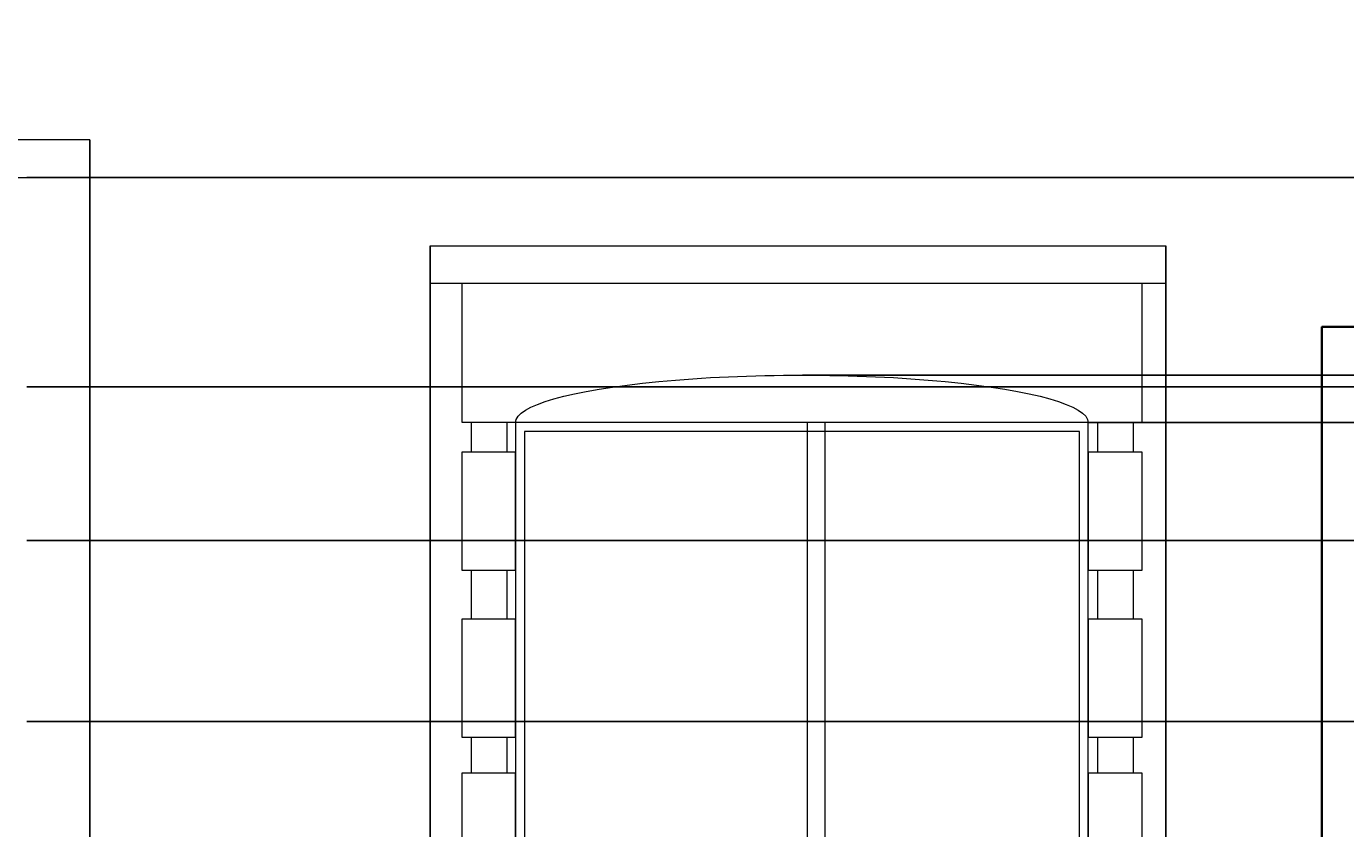
# Model space of a CAD drawing. Units: inches. Extents: x 69 to 650, y -16 to 573.
# Tile 20 of 26: x 383 to 531, y 308 to 398. Entities that reach past the tile are written whole.
import ezdxf

# ---------------------------------------------------------------- set-up
doc = ezdxf.new("R2010")
doc.units = ezdxf.units.IN
doc.header["$MEASUREMENT"] = 0
for name, color, linetype, lineweight in [('A-ANNO-DIMS', 2, 'Continuous', 18), ('A-GLAZ', 4, 'Continuous', 18), ('A-WALL', 7, 'Continuous', 35)]:
    doc.layers.add(name, color=color, linetype=linetype, lineweight=lineweight)
doc.styles.get("Standard").update_dxf_attribs({"font": 'arial.ttf'})
doc.dimstyles.get("Standard").update_dxf_attribs({"dimtxt": 0.8125, "dimasz": 0.18, "dimexe": 0.18, "dimexo": 0.0625, "dimgap": 0.09, "dimtad": 0, "dimtih": 1, "dimtoh": 1, "dimdec": 4, "dimzin": 0, "dimdsep": 46, "dimlunit": 4, "dimtxsty": 'Standard', "dimcen": 0.09, "dimadec": 0, "dimazin": 0, "dimtfac": 1, "dimtdec": 4, "dimtofl": 0, "dimtmove": 0, "dimatfit": 3, "dimfxl": 1, "dimtolj": 1, "dimtzin": 0, "dimarcsym": 0})

# ---------------------------------------------------------------- blocks, each defined once
blk = doc.blocks.new('WIN-ARCH-SURROUND')
for p, q in [((0, 129.06), (0, 124.83)), ((82.63, 129.06), (0, 129.06)), ((82.63, 124.83), (82.63, 129.06)), ((0, 124.83), (82.63, 124.83)), ((2.69, 109.21), (2.69, 124.83)), ((79.05, 109.21), (79.05, 124.83)), ((3.69, 109.21), (2.69, 109.21)), ((3.69, 109.21), (3.69, 105.89)), ((3.69, 109.21), (78.05, 109.21)), ((7.69, 109.21), (7.69, 105.89)), ((8.73, 105.89), (8.73, 109.21)), ((38.31, 109.21), (38.31, 38)), ((40.31, 109.21), (40.31, 38)), ((74.05, 109.21), (74.05, 105.89)), ((78.05, 109.21), (79.05, 109.21)), ((78.05, 109.21), (78.05, 105.89)), ((3.69, 92.64), (3.69, 87.15)), ((7.69, 92.64), (7.69, 87.15)), ((74.05, 92.64), (74.05, 87.15)), ((78.05, 92.64), (78.05, 87.15)), ((3.69, 73.9), (3.69, 69.84)), ((7.69, 73.9), (7.69, 69.84)), ((74.05, 73.9), (74.05, 69.84)), ((78.05, 73.9), (78.05, 69.84)), ((3.69, 56.59), (3.69, 51.51)), ((7.69, 56.59), (7.69, 51.51)), ((74.05, 56.59), (74.05, 51.51)), ((78.05, 56.59), (78.05, 51.51)), ((3.69, 38.26), (3.69, 33.16)), ((7.69, 38.26), (7.69, 33.16)), ((74.05, 38.26), (74.05, 33.16)), ((78.05, 38.26), (78.05, 33.16)), ((3.69, 19.91), (3.69, 0)), ((7.69, 19.91), (7.69, 0)), ((74.05, 19.91), (74.05, 0)), ((78.05, 19.91), (78.05, 0))]:
    blk.add_line(p, q)
for points in [[(8.73, 109.21), (73.05, 109.21), (73.05, 38.26), (8.73, 38.26)], [(9.73, 108.21), (72.05, 108.21), (72.05, 39.26), (9.73, 39.26)], [(2.69, 105.89), (8.73, 105.89), (8.73, 92.64), (2.69, 92.64)], [(73.05, 105.89), (79.1, 105.89), (79.1, 92.64), (73.05, 92.64)], [(2.69, 87.15), (8.73, 87.15), (8.73, 73.9), (2.69, 73.9)], [(73.05, 87.15), (79.1, 87.15), (79.1, 73.9), (73.05, 73.9)], [(2.69, 69.84), (8.73, 69.84), (8.73, 56.59), (2.69, 56.59)], [(73.05, 69.84), (79.1, 69.84), (79.1, 56.59), (73.05, 56.59)], [(2.69, 51.51), (8.73, 51.51), (8.73, 38.26), (2.69, 38.26)], [(73.05, 51.51), (79.1, 51.51), (79.1, 38.26), (73.05, 38.26)], [(2.65, 33.16), (8.69, 33.16), (8.69, 19.91), (2.65, 19.91)], [(73.01, 33.16), (79.06, 33.16), (79.06, 19.91), (73.01, 19.91)]]:
    blk.add_lwpolyline(points, close=True)
blk.add_ellipse((40.89, 109.21), major_axis=(32.16, 0), ratio=0.165597, start_param=6.283185, end_param=9.424778)
blk = doc.blocks.new('*D19')
at = {"layer": 'A-ANNO-DIMS', "color": 0, "lineweight": -2, "transparency": 16777216}
for p, q in [((99.56, 471.72), (99.56, 572.74)), ((99.74, 572.56), (358.57, 572.56)), ((619.38, 572.56), (360.54, 572.56)), ((619.56, 87.99), (619.56, 572.74))]:
    blk.add_line(p, q, dxfattribs=at)
at = {"layer": 'A-ANNO-DIMS', "color": 0, "transparency": 16777216}
for points in [[(99.74, 572.59), (99.74, 572.53), (99.56, 572.56)], [(619.38, 572.59), (619.38, 572.53), (619.56, 572.56)]]:
    blk.add_solid(points, dxfattribs=at)
at = {"layer": 'Defpoints', "color": 0, "transparency": 16777216}
for p in [(619.56, 572.56), (99.56, 471.66), (619.56, 87.93)]:
    blk.add_point(p, dxfattribs=at)
at = {"layer": 'A-ANNO-DIMS', "color": 0, "transparency": 16777216, "insert": (359.56, 572.56), "char_height": 0.812, "attachment_point": 5}
blk.add_mtext('\\A1;520', dxfattribs=at)
blk = doc.blocks.new('*D20')
at = {"layer": 'A-ANNO-DIMS', "color": 0, "lineweight": -2, "transparency": 16777216}
for p, q in [((504.24, 544.16), (648.14, 544.16)), ((647.96, 543.98), (647.96, 304.55)), ((647.96, 64.11), (647.96, 303.54)), ((619.62, 63.93), (648.14, 63.93))]:
    blk.add_line(p, q, dxfattribs=at)
at = {"layer": 'A-ANNO-DIMS', "color": 0, "transparency": 16777216}
for points in [[(647.93, 543.98), (647.99, 543.98), (647.96, 544.16)], [(647.93, 64.11), (647.99, 64.11), (647.96, 63.93)]]:
    blk.add_solid(points, dxfattribs=at)
at = {"layer": 'Defpoints', "color": 0, "transparency": 16777216}
for p in [(504.18, 544.16), (647.96, 544.16), (619.56, 63.93)]:
    blk.add_point(p, dxfattribs=at)
at = {"layer": 'A-ANNO-DIMS', "color": 0, "transparency": 16777216, "insert": (647.96, 304.04), "char_height": 0.812, "attachment_point": 5}
blk.add_mtext('\\A1;480.2', dxfattribs=at)
blk = doc.blocks.new('*D38')
at = {"layer": 'A-ANNO-DIMS', "color": 0, "lineweight": -2, "transparency": 16777216}
for p, q in [((307.8, 384.84), (307.8, 35.35)), ((390.43, 384.84), (390.43, 35.35)), ((307.98, 35.53), (347.65, 35.53)), ((390.25, 35.53), (350.57, 35.53))]:
    blk.add_line(p, q, dxfattribs=at)
at = {"layer": 'A-ANNO-DIMS', "color": 0, "transparency": 16777216}
for points in [[(307.98, 35.56), (307.98, 35.5), (307.8, 35.53)], [(390.25, 35.56), (390.25, 35.5), (390.43, 35.53)]]:
    blk.add_solid(points, dxfattribs=at)
at = {"layer": 'Defpoints', "color": 0, "transparency": 16777216}
for p in [(307.8, 384.9), (390.43, 384.9), (390.43, 35.53)]:
    blk.add_point(p, dxfattribs=at)
at = {"layer": 'A-ANNO-DIMS', "color": 0, "transparency": 16777216, "insert": (349.11, 35.53), "char_height": 0.812, "attachment_point": 5}
blk.add_mtext('\\A1;82.63', dxfattribs=at)
blk = doc.blocks.new('*D39')
at = {"layer": 'A-ANNO-DIMS', "color": 0, "lineweight": -2, "transparency": 16777216}
for p, q in [((390.43, 384.84), (390.43, 35.35)), ((428.66, 372.93), (428.66, 35.35)), ((390.61, 35.53), (407.77, 35.53)), ((428.48, 35.53), (411.32, 35.53))]:
    blk.add_line(p, q, dxfattribs=at)
at = {"layer": 'A-ANNO-DIMS', "color": 0, "transparency": 16777216}
for points in [[(390.61, 35.56), (390.61, 35.5), (390.43, 35.53)], [(428.48, 35.56), (428.48, 35.5), (428.66, 35.53)]]:
    blk.add_solid(points, dxfattribs=at)
at = {"layer": 'Defpoints', "color": 0, "transparency": 16777216}
for p in [(390.43, 384.9), (428.66, 372.99), (428.66, 35.53)]:
    blk.add_point(p, dxfattribs=at)
at = {"layer": 'A-ANNO-DIMS', "color": 0, "transparency": 16777216, "insert": (409.55, 35.53), "char_height": 0.812, "attachment_point": 5}
blk.add_mtext('\\A1;38.236', dxfattribs=at)
blk = doc.blocks.new('*D40')
at = {"layer": 'A-ANNO-DIMS', "color": 0, "lineweight": -2, "transparency": 16777216}
for p, q in [((511.3, 372.93), (511.3, 35.35)), ((528.81, 243.87), (528.81, 35.35)), ((511.48, 35.53), (518.32, 35.53)), ((528.63, 35.53), (521.79, 35.53))]:
    blk.add_line(p, q, dxfattribs=at)
at = {"layer": 'A-ANNO-DIMS', "color": 0, "transparency": 16777216}
for points in [[(511.48, 35.56), (511.48, 35.5), (511.3, 35.53)], [(528.63, 35.56), (528.63, 35.5), (528.81, 35.53)]]:
    blk.add_solid(points, dxfattribs=at)
at = {"layer": 'Defpoints', "color": 0, "transparency": 16777216}
for p in [(511.3, 372.99), (528.81, 243.93), (528.81, 35.53)]:
    blk.add_point(p, dxfattribs=at)
at = {"layer": 'A-ANNO-DIMS', "color": 0, "transparency": 16777216, "insert": (520.06, 35.53), "char_height": 0.812, "attachment_point": 5}
blk.add_mtext('\\A1;17.514', dxfattribs=at)
blk = doc.blocks.new('*D43')
at = {"layer": 'A-ANNO-DIMS', "color": 0, "lineweight": -2, "transparency": 16777216}
for p, q in [((502.63, 353.14), (648.14, 353.14)), ((647.96, 352.96), (647.96, 318.17)), ((647.96, 282.37), (647.96, 317.16)), ((502.63, 282.19), (648.14, 282.19))]:
    blk.add_line(p, q, dxfattribs=at)
at = {"layer": 'A-ANNO-DIMS', "color": 0, "transparency": 16777216}
for points in [[(647.93, 352.96), (647.99, 352.96), (647.96, 353.14)], [(647.93, 282.37), (647.99, 282.37), (647.96, 282.19)]]:
    blk.add_solid(points, dxfattribs=at)
at = {"layer": 'Defpoints', "color": 0, "transparency": 16777216}
for p in [(502.56, 353.14), (647.96, 353.14), (502.56, 282.19)]:
    blk.add_point(p, dxfattribs=at)
at = {"layer": 'A-ANNO-DIMS', "color": 0, "transparency": 16777216, "insert": (647.96, 317.67), "char_height": 0.812, "attachment_point": 5}
blk.add_mtext('\\A1;70.95', dxfattribs=at)
blk = doc.blocks.new('*D44')
at = {"layer": 'A-ANNO-DIMS', "color": 0, "lineweight": -2, "transparency": 16777216}
for p, q in [((470.47, 358.46), (648.14, 358.46)), ((647.96, 358.28), (647.96, 356.31)), ((647.96, 353.32), (647.96, 355.3)), ((502.63, 353.14), (648.14, 353.14))]:
    blk.add_line(p, q, dxfattribs=at)
at = {"layer": 'A-ANNO-DIMS', "color": 0, "transparency": 16777216}
for points in [[(647.93, 358.28), (647.99, 358.28), (647.96, 358.46)], [(647.93, 353.32), (647.99, 353.32), (647.96, 353.14)]]:
    blk.add_solid(points, dxfattribs=at)
at = {"layer": 'Defpoints', "color": 0, "transparency": 16777216}
for p in [(470.41, 358.46), (647.96, 358.46), (502.56, 353.14)]:
    blk.add_point(p, dxfattribs=at)
at = {"layer": 'A-ANNO-DIMS', "color": 0, "transparency": 16777216, "insert": (647.96, 355.8), "char_height": 0.812, "attachment_point": 5}
blk.add_mtext('\\A1;5.325', dxfattribs=at)
blk = doc.blocks.new('*D73')
at = {"layer": 'A-ANNO-DIMS', "color": 0, "lineweight": -2, "transparency": 16777216}
for p, q in [((383.36, 319.57), (648.14, 319.57)), ((647.96, 319.39), (647.96, 302.7)), ((647.96, 284.99), (647.96, 301.69)), ((383.36, 284.81), (648.14, 284.81))]:
    blk.add_line(p, q, dxfattribs=at)
at = {"layer": 'A-ANNO-DIMS', "color": 0, "transparency": 16777216}
for points in [[(647.93, 319.39), (647.99, 319.39), (647.96, 319.57)], [(647.93, 284.99), (647.99, 284.99), (647.96, 284.81)]]:
    blk.add_solid(points, dxfattribs=at)
at = {"layer": 'Defpoints', "color": 0, "transparency": 16777216}
for p in [(383.3, 319.57), (647.96, 319.57), (383.3, 284.81)]:
    blk.add_point(p, dxfattribs=at)
at = {"layer": 'A-ANNO-DIMS', "color": 0, "transparency": 16777216, "insert": (647.96, 302.19), "char_height": 0.812, "attachment_point": 5}
blk.add_mtext('\\A1;34.76', dxfattribs=at)
blk = doc.blocks.new('*D74')
at = {"layer": 'A-ANNO-DIMS', "color": 0, "lineweight": -2, "transparency": 16777216}
for p, q in [((383.36, 339.91), (648.14, 339.91)), ((647.96, 339.73), (647.96, 330.25)), ((647.96, 319.75), (647.96, 329.23)), ((383.36, 319.57), (648.14, 319.57))]:
    blk.add_line(p, q, dxfattribs=at)
at = {"layer": 'A-ANNO-DIMS', "color": 0, "transparency": 16777216}
for points in [[(647.93, 339.73), (647.99, 339.73), (647.96, 339.91)], [(647.93, 319.75), (647.99, 319.75), (647.96, 319.57)]]:
    blk.add_solid(points, dxfattribs=at)
at = {"layer": 'Defpoints', "color": 0, "transparency": 16777216}
for p in [(383.3, 339.91), (647.96, 339.91), (383.3, 319.57)]:
    blk.add_point(p, dxfattribs=at)
at = {"layer": 'A-ANNO-DIMS', "color": 0, "transparency": 16777216, "insert": (647.96, 329.74), "char_height": 0.812, "attachment_point": 5}
blk.add_mtext('\\A1;20.332', dxfattribs=at)
blk = doc.blocks.new('*D75')
at = {"layer": 'A-ANNO-DIMS', "color": 0, "lineweight": -2, "transparency": 16777216}
for p, q in [((383.36, 357.16), (648.14, 357.16)), ((647.96, 356.98), (647.96, 349.04)), ((647.96, 340.09), (647.96, 348.03)), ((383.36, 339.91), (648.14, 339.91))]:
    blk.add_line(p, q, dxfattribs=at)
at = {"layer": 'A-ANNO-DIMS', "color": 0, "transparency": 16777216}
for points in [[(647.93, 356.98), (647.99, 356.98), (647.96, 357.16)], [(647.93, 340.09), (647.99, 340.09), (647.96, 339.91)]]:
    blk.add_solid(points, dxfattribs=at)
at = {"layer": 'Defpoints', "color": 0, "transparency": 16777216}
for p in [(383.3, 357.16), (647.96, 357.16), (383.3, 339.91)]:
    blk.add_point(p, dxfattribs=at)
at = {"layer": 'A-ANNO-DIMS', "color": 0, "transparency": 16777216, "insert": (647.96, 348.53), "char_height": 0.812, "attachment_point": 5}
blk.add_mtext('\\A1;17.254', dxfattribs=at)
blk = doc.blocks.new('*D76')
at = {"layer": 'A-ANNO-DIMS', "color": 0, "lineweight": -2, "transparency": 16777216}
for p, q in [((383.36, 380.67), (648.14, 380.67)), ((647.96, 380.49), (647.96, 369.42)), ((647.96, 357.34), (647.96, 368.41)), ((383.36, 357.16), (648.14, 357.16))]:
    blk.add_line(p, q, dxfattribs=at)
at = {"layer": 'A-ANNO-DIMS', "color": 0, "transparency": 16777216}
for points in [[(647.93, 380.49), (647.99, 380.49), (647.96, 380.67)], [(647.93, 357.34), (647.99, 357.34), (647.96, 357.16)]]:
    blk.add_solid(points, dxfattribs=at)
at = {"layer": 'Defpoints', "color": 0, "transparency": 16777216}
for p in [(383.3, 380.67), (647.96, 380.67), (383.3, 357.16)]:
    blk.add_point(p, dxfattribs=at)
at = {"layer": 'A-ANNO-DIMS', "color": 0, "transparency": 16777216, "insert": (647.96, 368.92), "char_height": 0.812, "attachment_point": 5}
blk.add_mtext('\\A1;23.51', dxfattribs=at)

msp = doc.modelspace()

# ---------------------------------------------------------------- linework, layer by layer
at = {"layer": 'A-GLAZ'}
for p, q in [((390.4291, 384.8986), (307.7955, 384.8986)), ((390.4291, 384.8986), (390.4291, 380.6715)), ((307.7955, 380.6715), (390.4291, 380.6715))]:
    msp.add_line(p, q, dxfattribs=at)
at = {"layer": 'A-WALL'}
msp.add_lwpolyline([(619.555, 363.8739), (528.812, 363.8739), (528.812, 243.93), (619.555, 243.93)], close=True, dxfattribs=at)

# ---------------------------------------------------------------- block references
at = {"layer": 'A-GLAZ', "extrusion": (0, 0, -1), "zscale": -1}
msp.add_blockref('WIN-ARCH-SURROUND', (-511.298, 243.93), dxfattribs=at)

# ---------------------------------------------------------------- dimensions: what is measured, and where the dimension line sits
at = {"layer": 'A-ANNO-DIMS'}
for base, p1, p2, override, picture, middle in [((619.555, 572.5573), (99.556, 471.6595), (619.555, 87.93), {"dimdec": 0, "dimlfac": 1, "dimrnd": 0, "dimzin": 0, "dimdsep": 46, "dimlunit": 2}, '*D19', (359.5555, 572.5573)), ((390.4291, 35.53), (307.7955, 384.8986), (390.4291, 384.8986), {"dimdec": 2, "dimlfac": 1, "dimrnd": 0, "dimzin": 0, "dimdsep": 46, "dimlunit": 2}, '*D38', (349.1123, 35.53)), ((428.6648, 35.53), (390.4291, 384.8986), (428.6648, 372.9907), {"dimdec": 3, "dimlfac": 1, "dimrnd": 0, "dimzin": 0, "dimdsep": 46, "dimlunit": 2}, '*D39', (409.547, 35.53)), ((528.812, 35.53), (511.2984, 372.9907), (528.812, 243.93), {"dimdec": 3, "dimlfac": 1, "dimrnd": 0, "dimzin": 0, "dimdsep": 46, "dimlunit": 2}, '*D40', (520.0552, 35.53))]:
    dim = msp.add_linear_dim(base=base, p1=p1, p2=p2, dimstyle='Standard', override=override, dxfattribs=at)
    dim.commit()
    dim.dimension.update_dxf_attribs({"geometry": picture, "text_midpoint": middle})
for base, p1, p2, override, picture, middle in [((647.955, 544.1573), (619.555, 63.93), (504.1763, 544.1573), {"dimdec": 1, "dimlfac": 1, "dimrnd": 0, "dimzin": 0, "dimdsep": 46, "dimlunit": 2}, '*D20', (647.955, 304.0436)), ((647.955, 380.6715), (383.3022, 357.1599), (383.3022, 380.6715), {"dimdec": 2, "dimlfac": 1, "dimrnd": 0, "dimzin": 0, "dimdsep": 46, "dimlunit": 2}, '*D76', (647.955, 368.9157)), ((647.955, 357.1599), (383.3022, 339.9061), (383.3022, 357.1599), {"dimdec": 3, "dimlfac": 1, "dimrnd": 0, "dimzin": 0, "dimdsep": 46, "dimlunit": 2}, '*D75', (647.955, 348.533)), ((647.955, 358.4634), (502.5637, 353.1381), (470.4053, 358.4634), {"dimdec": 3, "dimlfac": 1, "dimrnd": 0, "dimzin": 0, "dimdsep": 46, "dimlunit": 2}, '*D44', (647.955, 355.8008)), ((647.955, 353.1381), (502.5637, 282.1923), (502.5637, 353.1381), {"dimdec": 2, "dimlfac": 1, "dimrnd": 0, "dimzin": 0, "dimdsep": 46, "dimlunit": 2}, '*D43', (647.955, 317.6652)), ((647.955, 339.9061), (383.3022, 319.5737), (383.3022, 339.9061), {"dimdec": 3, "dimlfac": 1, "dimrnd": 0, "dimzin": 0, "dimdsep": 46, "dimlunit": 2}, '*D74', (647.955, 329.7399)), ((647.955, 319.5737), (383.3022, 284.812), (383.3022, 319.5737), {"dimdec": 2, "dimlfac": 1, "dimrnd": 0, "dimzin": 0, "dimdsep": 46, "dimlunit": 2}, '*D73', (647.955, 302.1928))]:
    dim = msp.add_linear_dim(base=base, p1=p1, p2=p2, angle=90, dimstyle='Standard', override=override, dxfattribs=at)
    dim.commit()
    dim.dimension.update_dxf_attribs({"geometry": picture, "text_midpoint": middle})

doc.saveas('drawing.dxf')
